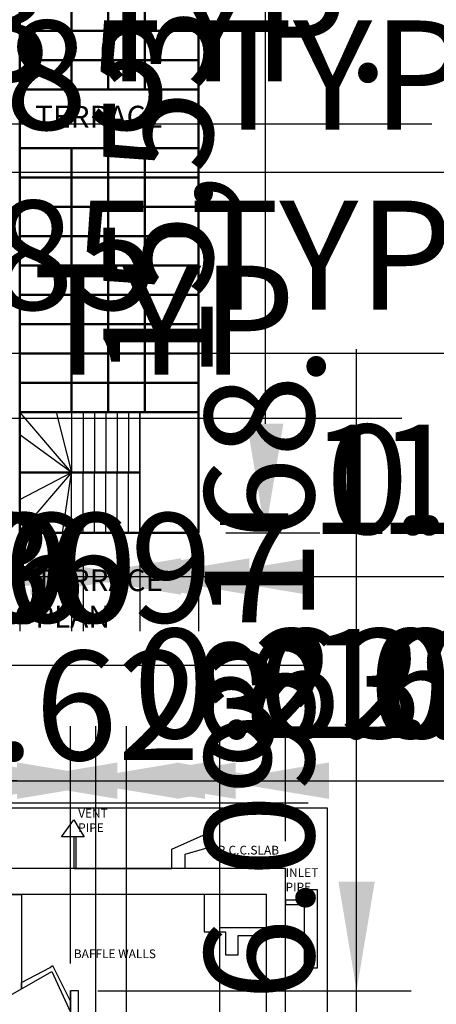
# Model space of a CAD drawing. Units: metres. Extents: x 782 to 1487, y 1262 to 7446.
# Tile 15 of 25: x 840.09 to 849.63, y 1279.51 to 1302.06. Entities that reach past the tile are written whole.
import ezdxf

# ---------------------------------------------------------------- set-up
doc = ezdxf.new("R2010")
doc.units = ezdxf.units.M
for name, color, linetype, lineweight in [('A-ANNO-DIMS', 2, 'Continuous', 18), ('A-ANNO-TEXT', 3, 'Continuous', 18), ('A-AREA-IDEN', 3, 'Continuous', 18), ('A-DETL', 7, 'Continuous', 25), ('A-FLOR-STRS', 3, 'Continuous', 25), ('A-WALL', 7, 'Continuous', 50)]:
    doc.layers.add(name, color=color, linetype=linetype, lineweight=lineweight)
doc.styles.get("Standard").update_dxf_attribs({"font": 'arial.ttf'})
doc.dimstyles.new('ISO-25', dxfattribs={"dimtxt": 2.5, "dimasz": 2.5, "dimexe": 1.25, "dimexo": 0.625, "dimtad": 1, "dimtxsty": 'Standard', "dimcen": 2.5, "dimadec": 0, "dimazin": 0, "dimtfac": 1, "dimtmove": 0, "dimatfit": 3, "dimfxl": 1, "dimarcsym": 0})

# ---------------------------------------------------------------- blocks, each defined once
blk = doc.blocks.new('*D8')
at = {"layer": 'A-ANNO-DIMS', "color": 0, "lineweight": -2, "transparency": 16777216}
for p, q in [((844.81, 1305.835), (846.96, 1305.835)), ((845.71, 1303.335), (845.71, 1292.805)), ((844.81, 1290.305), (846.96, 1290.305))]:
    blk.add_line(p, q, dxfattribs=at)
at = {"layer": 'A-ANNO-DIMS', "color": 0, "transparency": 16777216}
for points in [[(845.293, 1303.335), (846.126, 1303.335), (845.71, 1305.835)], [(845.293, 1292.805), (846.126, 1292.805), (845.71, 1290.305)]]:
    blk.add_solid(points, dxfattribs=at)
at = {"layer": 'Defpoints', "color": 0, "transparency": 16777216}
for p in [(844.185, 1305.835), (844.185, 1290.305), (845.71, 1290.305)]:
    blk.add_point(p, dxfattribs=at)
at = {"layer": 'A-ANNO-DIMS', "color": 0, "transparency": 16777216, "insert": (843.582, 1298.07), "char_height": 2.5, "attachment_point": 5, "rotation": 90}
blk.add_mtext('15,53', dxfattribs=at)
blk = doc.blocks.new('*D21')
at = {"layer": 'A-ANNO-DIMS', "color": 0, "lineweight": -2, "transparency": 16777216}
for p, q in [((827.576, 1298.565), (825.076, 1298.565)), ((830.076, 1298.565), (830.923, 1298.565)), ((833.423, 1298.565), (852.255, 1298.565)), ((830.076, 1298.073), (830.076, 1297.315)), ((830.923, 1298.073), (830.923, 1297.315))]:
    blk.add_line(p, q, dxfattribs=at)
at = {"layer": 'A-ANNO-DIMS', "color": 0, "transparency": 16777216}
for points in [[(827.576, 1298.981), (827.576, 1298.148), (830.076, 1298.565)], [(833.423, 1298.981), (833.423, 1298.148), (830.923, 1298.565)]]:
    blk.add_solid(points, dxfattribs=at)
at = {"layer": 'Defpoints', "color": 0, "transparency": 16777216}
for p in [(830.076, 1298.698), (830.923, 1298.698), (830.923, 1298.565)]:
    blk.add_point(p, dxfattribs=at)
at = {"layer": 'A-ANNO-DIMS', "color": 0, "transparency": 16777216, "insert": (844.089, 1300.466), "char_height": 2.5, "attachment_point": 5}
blk.add_mtext('0.85 TYP.', dxfattribs=at)
blk = doc.blocks.new('*D22')
at = {"layer": 'A-ANNO-DIMS', "color": 0, "lineweight": -2, "transparency": 16777216}
for p, q in [((812.79, 1292.934), (810.29, 1292.934)), ((815.29, 1292.934), (816.179, 1292.934)), ((818.679, 1292.934), (848.834, 1292.934)), ((815.29, 1292.442), (815.29, 1291.684)), ((816.179, 1292.442), (816.179, 1291.684))]:
    blk.add_line(p, q, dxfattribs=at)
at = {"layer": 'A-ANNO-DIMS', "color": 0, "transparency": 16777216}
for points in [[(812.79, 1293.351), (812.79, 1292.517), (815.29, 1292.934)], [(818.679, 1293.351), (818.679, 1292.517), (816.179, 1292.934)]]:
    blk.add_solid(points, dxfattribs=at)
at = {"layer": 'Defpoints', "color": 0, "transparency": 16777216}
for p in [(815.29, 1293.067), (816.179, 1293.067), (816.179, 1292.934)]:
    blk.add_point(p, dxfattribs=at)
at = {"layer": 'A-ANNO-DIMS', "color": 0, "transparency": 16777216, "insert": (835.007, 1294.852), "char_height": 2.5, "attachment_point": 5}
blk.add_mtext('DOOR 0.89 TYP.', dxfattribs=at)
blk = doc.blocks.new('*D24')
at = {"layer": 'A-ANNO-DIMS', "color": 0, "lineweight": -2, "transparency": 16777216}
for p, q in [((811.209, 1294.423), (808.709, 1294.423)), ((813.709, 1294.423), (814.559, 1294.423)), ((817.059, 1294.423), (852.649, 1294.423)), ((813.709, 1293.926), (813.709, 1293.173)), ((814.559, 1293.926), (814.559, 1293.173))]:
    blk.add_line(p, q, dxfattribs=at)
at = {"layer": 'A-ANNO-DIMS', "color": 0, "transparency": 16777216}
for points in [[(811.209, 1294.84), (811.209, 1294.006), (813.709, 1294.423)], [(817.059, 1294.84), (817.059, 1294.006), (814.559, 1294.423)]]:
    blk.add_solid(points, dxfattribs=at)
at = {"layer": 'Defpoints', "color": 0, "transparency": 16777216}
for p in [(813.709, 1294.551), (814.559, 1294.551), (814.559, 1294.423)]:
    blk.add_point(p, dxfattribs=at)
at = {"layer": 'A-ANNO-DIMS', "color": 0, "transparency": 16777216, "insert": (836.104, 1296.342), "char_height": 2.5, "attachment_point": 5}
blk.add_mtext('DOOR D2 0.85 TYP.', dxfattribs=at)
blk = doc.blocks.new('*D27')
at = {"layer": 'A-ANNO-DIMS', "color": 0, "lineweight": -2, "transparency": 16777216}
for p, q in [((825.463, 1299.672), (822.963, 1299.672)), ((827.963, 1299.672), (828.193, 1299.672)), ((830.693, 1299.672), (849.525, 1299.672)), ((827.963, 1299.184), (827.963, 1298.422)), ((828.193, 1299.184), (828.193, 1298.422))]:
    blk.add_line(p, q, dxfattribs=at)
at = {"layer": 'A-ANNO-DIMS', "color": 0, "transparency": 16777216}
for points in [[(825.463, 1300.088), (825.463, 1299.255), (827.963, 1299.672)], [(830.693, 1300.088), (830.693, 1299.255), (828.193, 1299.672)]]:
    blk.add_solid(points, dxfattribs=at)
at = {"layer": 'Defpoints', "color": 0, "transparency": 16777216}
for p in [(827.963, 1299.809), (828.193, 1299.809), (828.193, 1299.672)]:
    blk.add_point(p, dxfattribs=at)
at = {"layer": 'A-ANNO-DIMS', "color": 0, "transparency": 16777216, "insert": (841.359, 1301.574), "char_height": 2.5, "attachment_point": 5}
blk.add_mtext('0.23 TYP.', dxfattribs=at)
blk = doc.blocks.new('*D97')
at = {"layer": 'A-ANNO-DIMS', "color": 0, "lineweight": -2, "transparency": 16777216}
for p, q in [((827.962, 1289.68), (827.962, 1286.027)), ((829.151, 1289.68), (829.151, 1286.027)), ((825.462, 1287.277), (822.962, 1287.277)), ((827.962, 1287.277), (829.151, 1287.277)), ((831.651, 1287.277), (841.665, 1287.277))]:
    blk.add_line(p, q, dxfattribs=at)
at = {"layer": 'A-ANNO-DIMS', "color": 0, "transparency": 16777216}
for points in [[(825.462, 1287.694), (825.462, 1286.861), (827.962, 1287.277)], [(831.651, 1287.694), (831.651, 1286.861), (829.151, 1287.277)]]:
    blk.add_solid(points, dxfattribs=at)
at = {"layer": 'Defpoints', "color": 0, "transparency": 16777216}
for p in [(827.962, 1290.305), (829.151, 1290.305), (829.151, 1287.277)]:
    blk.add_point(p, dxfattribs=at)
at = {"layer": 'A-ANNO-DIMS', "color": 0, "transparency": 16777216, "insert": (837.908, 1289.179), "char_height": 2.5, "attachment_point": 5}
blk.add_mtext('1.19', dxfattribs=at)
blk = doc.blocks.new('*D98')
at = {"layer": 'A-ANNO-DIMS', "color": 0, "lineweight": -2, "transparency": 16777216}
for p, q in [((829.151, 1289.68), (829.151, 1286.027)), ((829.412, 1289.68), (829.412, 1286.027)), ((826.651, 1287.277), (824.151, 1287.277)), ((829.151, 1287.277), (829.412, 1287.277)), ((831.912, 1287.277), (842.154, 1287.277))]:
    blk.add_line(p, q, dxfattribs=at)
at = {"layer": 'A-ANNO-DIMS', "color": 0, "transparency": 16777216}
for points in [[(826.651, 1287.694), (826.651, 1286.861), (829.151, 1287.277)], [(831.912, 1287.694), (831.912, 1286.861), (829.412, 1287.277)]]:
    blk.add_solid(points, dxfattribs=at)
at = {"layer": 'Defpoints', "color": 0, "transparency": 16777216}
for p in [(829.151, 1290.305), (829.412, 1290.305), (829.412, 1287.277)]:
    blk.add_point(p, dxfattribs=at)
at = {"layer": 'A-ANNO-DIMS', "color": 0, "transparency": 16777216, "insert": (838.283, 1289.179), "char_height": 2.5, "attachment_point": 5}
blk.add_mtext('0.26', dxfattribs=at)
blk = doc.blocks.new('*D99')
at = {"layer": 'A-ANNO-DIMS', "color": 0, "lineweight": -2, "transparency": 16777216}
for p, q in [((829.412, 1289.68), (829.412, 1286.027)), ((830.716, 1289.68), (830.716, 1286.027)), ((826.912, 1287.277), (824.412, 1287.277)), ((829.412, 1287.277), (830.716, 1287.277)), ((833.216, 1287.277), (843.216, 1287.277))]:
    blk.add_line(p, q, dxfattribs=at)
at = {"layer": 'A-ANNO-DIMS', "color": 0, "transparency": 16777216}
for points in [[(826.912, 1287.694), (826.912, 1286.861), (829.412, 1287.277)], [(833.216, 1287.694), (833.216, 1286.861), (830.716, 1287.277)]]:
    blk.add_solid(points, dxfattribs=at)
at = {"layer": 'Defpoints', "color": 0, "transparency": 16777216}
for p in [(829.412, 1290.305), (830.716, 1290.305), (830.716, 1287.277)]:
    blk.add_point(p, dxfattribs=at)
at = {"layer": 'A-ANNO-DIMS', "color": 0, "transparency": 16777216, "insert": (839.466, 1289.18), "char_height": 2.5, "attachment_point": 5}
blk.add_mtext('1.30', dxfattribs=at)
blk = doc.blocks.new('*D100')
at = {"layer": 'A-ANNO-DIMS', "color": 0, "lineweight": -2, "transparency": 16777216}
for p, q in [((830.716, 1289.68), (830.716, 1286.027)), ((832.412, 1289.68), (832.412, 1286.027)), ((828.216, 1287.277), (825.716, 1287.277)), ((830.716, 1287.277), (832.412, 1287.277)), ((834.912, 1287.277), (846.863, 1287.277))]:
    blk.add_line(p, q, dxfattribs=at)
at = {"layer": 'A-ANNO-DIMS', "color": 0, "transparency": 16777216}
for points in [[(828.216, 1287.694), (828.216, 1286.861), (830.716, 1287.277)], [(834.912, 1287.694), (834.912, 1286.861), (832.412, 1287.277)]]:
    blk.add_solid(points, dxfattribs=at)
at = {"layer": 'Defpoints', "color": 0, "transparency": 16777216}
for p in [(830.716, 1290.305), (832.412, 1290.305), (832.412, 1287.277)]:
    blk.add_point(p, dxfattribs=at)
at = {"layer": 'A-ANNO-DIMS', "color": 0, "transparency": 16777216, "insert": (842.138, 1289.179), "char_height": 2.5, "attachment_point": 5}
blk.add_mtext('1.697', dxfattribs=at)
blk = doc.blocks.new('*D105')
at = {"layer": 'A-ANNO-DIMS', "color": 0, "lineweight": -2, "transparency": 16777216}
for p, q in [((840.091, 1289.68), (840.091, 1288.055)), ((841.28, 1289.68), (841.28, 1288.055)), ((837.591, 1289.305), (835.091, 1289.305)), ((840.091, 1289.305), (841.28, 1289.305)), ((843.78, 1289.305), (853.794, 1289.305))]:
    blk.add_line(p, q, dxfattribs=at)
at = {"layer": 'A-ANNO-DIMS', "color": 0, "transparency": 16777216}
for points in [[(837.591, 1289.722), (837.591, 1288.889), (840.091, 1289.305)], [(843.78, 1289.722), (843.78, 1288.889), (841.28, 1289.305)]]:
    blk.add_solid(points, dxfattribs=at)
at = {"layer": 'Defpoints', "color": 0, "transparency": 16777216}
for p in [(840.091, 1290.305), (841.28, 1290.305), (841.28, 1289.305)]:
    blk.add_point(p, dxfattribs=at)
at = {"layer": 'A-ANNO-DIMS', "color": 0, "transparency": 16777216, "insert": (850.037, 1291.207), "char_height": 2.5, "attachment_point": 5}
blk.add_mtext('1.19', dxfattribs=at)
blk = doc.blocks.new('*D106')
at = {"layer": 'A-ANNO-DIMS', "color": 0, "lineweight": -2, "transparency": 16777216}
for p, q in [((841.28, 1289.68), (841.28, 1288.055)), ((841.541, 1289.68), (841.541, 1288.055)), ((838.78, 1289.305), (836.28, 1289.305)), ((841.28, 1289.305), (841.541, 1289.305)), ((844.041, 1289.305), (854.283, 1289.305))]:
    blk.add_line(p, q, dxfattribs=at)
at = {"layer": 'A-ANNO-DIMS', "color": 0, "transparency": 16777216}
for points in [[(838.78, 1289.722), (838.78, 1288.889), (841.28, 1289.305)], [(844.041, 1289.722), (844.041, 1288.889), (841.541, 1289.305)]]:
    blk.add_solid(points, dxfattribs=at)
at = {"layer": 'Defpoints', "color": 0, "transparency": 16777216}
for p in [(841.28, 1290.305), (841.541, 1290.305), (841.541, 1289.305)]:
    blk.add_point(p, dxfattribs=at)
at = {"layer": 'A-ANNO-DIMS', "color": 0, "transparency": 16777216, "insert": (850.412, 1291.207), "char_height": 2.5, "attachment_point": 5}
blk.add_mtext('0.26', dxfattribs=at)
blk = doc.blocks.new('*D107')
at = {"layer": 'A-ANNO-DIMS', "color": 0, "lineweight": -2, "transparency": 16777216}
for p, q in [((841.541, 1289.68), (841.541, 1288.055)), ((842.844, 1289.68), (842.844, 1288.055)), ((839.041, 1289.305), (836.541, 1289.305)), ((841.541, 1289.305), (842.844, 1289.305)), ((845.344, 1289.305), (855.344, 1289.305))]:
    blk.add_line(p, q, dxfattribs=at)
at = {"layer": 'A-ANNO-DIMS', "color": 0, "transparency": 16777216}
for points in [[(839.041, 1289.722), (839.041, 1288.889), (841.541, 1289.305)], [(845.344, 1289.722), (845.344, 1288.889), (842.844, 1289.305)]]:
    blk.add_solid(points, dxfattribs=at)
at = {"layer": 'Defpoints', "color": 0, "transparency": 16777216}
for p in [(841.541, 1290.305), (842.844, 1290.305), (842.844, 1289.305)]:
    blk.add_point(p, dxfattribs=at)
at = {"layer": 'A-ANNO-DIMS', "color": 0, "transparency": 16777216, "insert": (851.594, 1291.208), "char_height": 2.5, "attachment_point": 5}
blk.add_mtext('1.30', dxfattribs=at)
blk = doc.blocks.new('*D108')
at = {"layer": 'A-ANNO-DIMS', "color": 0, "lineweight": -2, "transparency": 16777216}
for p, q in [((842.844, 1289.68), (842.844, 1288.055)), ((844.185, 1289.68), (844.185, 1288.055)), ((840.344, 1289.305), (837.844, 1289.305)), ((842.844, 1289.305), (844.185, 1289.305)), ((846.685, 1289.305), (856.683, 1289.305))]:
    blk.add_line(p, q, dxfattribs=at)
at = {"layer": 'A-ANNO-DIMS', "color": 0, "transparency": 16777216}
for points in [[(840.344, 1289.722), (840.344, 1288.889), (842.844, 1289.305)], [(846.685, 1289.722), (846.685, 1288.889), (844.185, 1289.305)]]:
    blk.add_solid(points, dxfattribs=at)
at = {"layer": 'Defpoints', "color": 0, "transparency": 16777216}
for p in [(842.844, 1290.305), (844.185, 1290.305), (844.185, 1289.305)]:
    blk.add_point(p, dxfattribs=at)
at = {"layer": 'A-ANNO-DIMS', "color": 0, "transparency": 16777216, "insert": (852.934, 1291.208), "char_height": 2.5, "attachment_point": 5}
blk.add_mtext('1.34', dxfattribs=at)
blk = doc.blocks.new('*D148')
at = {"layer": 'A-ANNO-DIMS', "color": 0, "lineweight": -2, "transparency": 16777216}
for p, q in [((847.802, 1276.491), (847.802, 1288.69)), ((846.368, 1273.991), (849.052, 1273.991)), ((847.802, 1267.897), (847.802, 1273.991)), ((846.368, 1267.897), (849.052, 1267.897)), ((847.802, 1265.397), (847.802, 1262.897))]:
    blk.add_line(p, q, dxfattribs=at)
at = {"layer": 'A-ANNO-DIMS', "color": 0, "transparency": 16777216}
for points in [[(847.386, 1276.491), (848.219, 1276.491), (847.802, 1273.991)], [(847.386, 1265.397), (848.219, 1265.397), (847.802, 1267.897)]]:
    blk.add_solid(points, dxfattribs=at)
at = {"layer": 'Defpoints', "color": 0, "transparency": 16777216}
for p in [(845.743, 1273.991), (847.802, 1273.991), (845.743, 1267.897)]:
    blk.add_point(p, dxfattribs=at)
at = {"layer": 'A-ANNO-DIMS', "color": 0, "transparency": 16777216, "insert": (845.9, 1283.841), "char_height": 2.5, "attachment_point": 5, "rotation": 90}
blk.add_mtext('6.093', dxfattribs=at)
blk = doc.blocks.new('*D151')
at = {"layer": 'A-ANNO-DIMS', "color": 0, "lineweight": -2, "transparency": 16777216}
for p, q in [((839.686, 1273.694), (839.686, 1285.879)), ((841.835, 1273.694), (841.835, 1285.879)), ((837.186, 1284.629), (834.686, 1284.629)), ((839.686, 1284.629), (841.835, 1284.629)), ((844.335, 1284.629), (856.569, 1284.629))]:
    blk.add_line(p, q, dxfattribs=at)
at = {"layer": 'A-ANNO-DIMS', "color": 0, "transparency": 16777216}
for points in [[(837.186, 1285.046), (837.186, 1284.212), (839.686, 1284.629)], [(844.335, 1285.046), (844.335, 1284.212), (841.835, 1284.629)]]:
    blk.add_solid(points, dxfattribs=at)
at = {"layer": 'Defpoints', "color": 0, "transparency": 16777216}
for p in [(841.835, 1284.629), (839.686, 1273.069), (841.835, 1273.069)]:
    blk.add_point(p, dxfattribs=at)
at = {"layer": 'A-ANNO-DIMS', "color": 0, "transparency": 16777216, "insert": (851.702, 1286.531), "char_height": 2.5, "attachment_point": 5}
blk.add_mtext('2.149', dxfattribs=at)
blk = doc.blocks.new('*D152')
at = {"layer": 'A-ANNO-DIMS', "color": 0, "lineweight": -2, "transparency": 16777216}
for p, q in [((841.835, 1273.694), (841.835, 1285.879)), ((842.533, 1273.678), (842.533, 1285.879)), ((839.335, 1284.629), (836.835, 1284.629)), ((841.835, 1284.629), (842.533, 1284.629)), ((845.033, 1284.629), (855.269, 1284.629))]:
    blk.add_line(p, q, dxfattribs=at)
at = {"layer": 'A-ANNO-DIMS', "color": 0, "transparency": 16777216}
for points in [[(839.335, 1285.046), (839.335, 1284.212), (841.835, 1284.629)], [(845.033, 1285.046), (845.033, 1284.212), (842.533, 1284.629)]]:
    blk.add_solid(points, dxfattribs=at)
at = {"layer": 'Defpoints', "color": 0, "transparency": 16777216}
for p in [(842.533, 1284.629), (841.835, 1273.069), (842.533, 1273.053)]:
    blk.add_point(p, dxfattribs=at)
at = {"layer": 'A-ANNO-DIMS', "color": 0, "transparency": 16777216, "insert": (851.401, 1286.531), "char_height": 2.5, "attachment_point": 5}
blk.add_mtext('0.70', dxfattribs=at)
blk = doc.blocks.new('*D153')
at = {"layer": 'A-ANNO-DIMS', "color": 0, "lineweight": -2, "transparency": 16777216}
for p, q in [((842.533, 1273.678), (842.533, 1285.879)), ((844.669, 1273.698), (844.669, 1285.879)), ((840.033, 1284.629), (837.533, 1284.629)), ((842.533, 1284.629), (844.669, 1284.629)), ((847.169, 1284.629), (857.445, 1284.629))]:
    blk.add_line(p, q, dxfattribs=at)
at = {"layer": 'A-ANNO-DIMS', "color": 0, "transparency": 16777216}
for points in [[(840.033, 1285.046), (840.033, 1284.212), (842.533, 1284.629)], [(847.169, 1285.046), (847.169, 1284.212), (844.669, 1284.629)]]:
    blk.add_solid(points, dxfattribs=at)
at = {"layer": 'Defpoints', "color": 0, "transparency": 16777216}
for p in [(844.669, 1284.629), (842.533, 1273.053), (844.669, 1273.073)]:
    blk.add_point(p, dxfattribs=at)
at = {"layer": 'A-ANNO-DIMS', "color": 0, "transparency": 16777216, "insert": (853.557, 1286.509), "char_height": 2.5, "attachment_point": 5}
blk.add_mtext('2.14', dxfattribs=at)
blk = doc.blocks.new('*D156')
at = {"layer": 'A-ANNO-DIMS', "color": 0, "lineweight": -2, "transparency": 16777216}
for p, q in [((836.503, 1283.244), (836.503, 1285.879)), ((846.176, 1283.244), (846.176, 1285.879)), ((839.003, 1284.629), (843.676, 1284.629)), ((846.176, 1284.629), (858.362, 1284.629))]:
    blk.add_line(p, q, dxfattribs=at)
at = {"layer": 'A-ANNO-DIMS', "color": 0, "transparency": 16777216}
for points in [[(839.003, 1285.046), (839.003, 1284.212), (836.503, 1284.629)], [(843.676, 1285.046), (843.676, 1284.212), (846.176, 1284.629)]]:
    blk.add_solid(points, dxfattribs=at)
at = {"layer": 'Defpoints', "color": 0, "transparency": 16777216}
for p in [(846.176, 1284.629), (836.503, 1282.619), (846.176, 1282.619)]:
    blk.add_point(p, dxfattribs=at)
at = {"layer": 'A-ANNO-DIMS', "color": 0, "transparency": 16777216, "insert": (853.519, 1286.531), "char_height": 2.5, "attachment_point": 5}
blk.add_mtext('9.673', dxfattribs=at)
blk = doc.blocks.new('*D158')
at = {"layer": 'A-ANNO-DIMS', "color": 0, "lineweight": -2, "transparency": 16777216}
for p, q in [((836.503, 1283.244), (836.503, 1285.879)), ((837.132, 1282.644), (837.132, 1285.879)), ((834.003, 1284.629), (831.503, 1284.629)), ((836.503, 1284.629), (837.132, 1284.629)), ((839.632, 1284.629), (849.876, 1284.629))]:
    blk.add_line(p, q, dxfattribs=at)
at = {"layer": 'A-ANNO-DIMS', "color": 0, "transparency": 16777216}
for points in [[(834.003, 1285.046), (834.003, 1284.212), (836.503, 1284.629)], [(839.632, 1285.046), (839.632, 1284.212), (837.132, 1284.629)]]:
    blk.add_solid(points, dxfattribs=at)
at = {"layer": 'Defpoints', "color": 0, "transparency": 16777216}
for p in [(837.132, 1284.629), (836.503, 1282.619), (837.132, 1282.019)]:
    blk.add_point(p, dxfattribs=at)
at = {"layer": 'A-ANNO-DIMS', "color": 0, "transparency": 16777216, "insert": (846.004, 1286.531), "char_height": 2.5, "attachment_point": 5}
blk.add_mtext('0.63', dxfattribs=at)
blk = doc.blocks.new('*D159')
at = {"layer": 'A-ANNO-DIMS', "color": 0, "lineweight": -2, "transparency": 16777216}
for p, q in [((837.132, 1282.644), (837.132, 1285.879)), ((839.826, 1282.644), (839.826, 1285.879)), ((834.632, 1284.629), (832.132, 1284.629)), ((837.132, 1284.629), (839.826, 1284.629)), ((842.326, 1284.629), (854.545, 1284.629))]:
    blk.add_line(p, q, dxfattribs=at)
at = {"layer": 'A-ANNO-DIMS', "color": 0, "transparency": 16777216}
for points in [[(834.632, 1285.046), (834.632, 1284.212), (837.132, 1284.629)], [(842.326, 1285.046), (842.326, 1284.212), (839.826, 1284.629)]]:
    blk.add_solid(points, dxfattribs=at)
at = {"layer": 'Defpoints', "color": 0, "transparency": 16777216}
for p in [(839.826, 1284.629), (837.132, 1282.019), (839.826, 1282.019)]:
    blk.add_point(p, dxfattribs=at)
at = {"layer": 'A-ANNO-DIMS', "color": 0, "transparency": 16777216, "insert": (849.686, 1286.531), "char_height": 2.5, "attachment_point": 5}
blk.add_mtext('2.694', dxfattribs=at)
blk = doc.blocks.new('*D160')
at = {"layer": 'A-ANNO-DIMS', "color": 0, "lineweight": -2, "transparency": 16777216}
for p, q in [((839.826, 1280.313), (839.826, 1285.879)), ((841.255, 1280.444), (841.255, 1285.879)), ((837.326, 1284.629), (834.826, 1284.629)), ((839.826, 1284.629), (841.255, 1284.629)), ((843.755, 1284.629), (853.764, 1284.629))]:
    blk.add_line(p, q, dxfattribs=at)
at = {"layer": 'A-ANNO-DIMS', "color": 0, "transparency": 16777216}
for points in [[(837.326, 1285.046), (837.326, 1284.212), (839.826, 1284.629)], [(843.755, 1285.046), (843.755, 1284.212), (841.255, 1284.629)]]:
    blk.add_solid(points, dxfattribs=at)
at = {"layer": 'Defpoints', "color": 0, "transparency": 16777216}
for p in [(841.255, 1284.629), (841.255, 1279.819), (839.826, 1279.688)]:
    blk.add_point(p, dxfattribs=at)
at = {"layer": 'A-ANNO-DIMS', "color": 0, "transparency": 16777216, "insert": (850.01, 1286.531), "char_height": 2.5, "attachment_point": 5}
blk.add_mtext('1.43', dxfattribs=at)
blk = doc.blocks.new('*D161')
at = {"layer": 'A-ANNO-DIMS', "color": 0, "lineweight": -2, "transparency": 16777216}
for p, q in [((847.802, 1282.319), (847.802, 1294.509)), ((841.88, 1279.819), (849.052, 1279.819)), ((847.802, 1276.651), (847.802, 1279.819)), ((841.88, 1276.651), (849.052, 1276.651)), ((847.802, 1274.151), (847.802, 1271.651))]:
    blk.add_line(p, q, dxfattribs=at)
at = {"layer": 'A-ANNO-DIMS', "color": 0, "transparency": 16777216}
for points in [[(847.386, 1282.319), (848.219, 1282.319), (847.802, 1279.819)], [(847.386, 1274.151), (848.219, 1274.151), (847.802, 1276.651)]]:
    blk.add_solid(points, dxfattribs=at)
at = {"layer": 'Defpoints', "color": 0, "transparency": 16777216}
for p in [(841.255, 1279.819), (847.802, 1279.819), (841.255, 1276.651)]:
    blk.add_point(p, dxfattribs=at)
at = {"layer": 'A-ANNO-DIMS', "color": 0, "transparency": 16777216, "insert": (845.9, 1289.664), "char_height": 2.5, "attachment_point": 5, "rotation": 90}
blk.add_mtext('3.168', dxfattribs=at)
blk = doc.blocks.new('*D165')
at = {"layer": 'A-ANNO-DIMS', "color": 0, "lineweight": -2, "transparency": 16777216}
for p, q in [((826.388, 1283.885), (826.388, 1285.375)), ((832.011, 1283.885), (832.011, 1285.375)), ((823.888, 1284.125), (821.388, 1284.125)), ((826.388, 1284.125), (832.011, 1284.125)), ((834.511, 1284.125), (846.697, 1284.125))]:
    blk.add_line(p, q, dxfattribs=at)
at = {"layer": 'A-ANNO-DIMS', "color": 0, "transparency": 16777216}
for points in [[(823.888, 1284.541), (823.888, 1283.708), (826.388, 1284.125)], [(834.511, 1284.541), (834.511, 1283.708), (832.011, 1284.125)]]:
    blk.add_solid(points, dxfattribs=at)
at = {"layer": 'Defpoints', "color": 0, "transparency": 16777216}
for p in [(832.011, 1284.125), (826.388, 1283.26), (832.011, 1283.26)]:
    blk.add_point(p, dxfattribs=at)
at = {"layer": 'A-ANNO-DIMS', "color": 0, "transparency": 16777216, "insert": (841.854, 1286.027), "char_height": 2.5, "attachment_point": 5}
blk.add_mtext('5.623', dxfattribs=at)

msp = doc.modelspace()

# ---------------------------------------------------------------- linework, layer by layer
at = {"layer": 'A-DETL'}
for p, q in [((841.0475, 1283.3454), (841.3293, 1283.7291)), ((841.3293, 1283.7291), (841.4773, 1283.491)), ((841.3396, 1283.3454), (841.0475, 1283.3454)), ((841.3396, 1282.619), (841.3396, 1283.3454)), ((841.5677, 1283.3454), (841.3396, 1283.3454)), ((841.3807, 1282.619), (841.3807, 1283.3454)), ((841.4773, 1283.491), (841.5677, 1283.3454)), ((843.5698, 1283.0622), (844.4285, 1283.4455)), ((844.4285, 1283.4455), (844.4285, 1283.0987)), ((843.5698, 1282.619), (843.5698, 1283.0622)), ((844.4285, 1283.0987), (843.8731, 1282.9355)), ((843.8731, 1282.9355), (843.8731, 1282.619)), ((841.3396, 1282.619), (843.5698, 1282.619)), ((841.3396, 1282.619), (841.5184, 1282.619)), ((841.5184, 1282.619), (841.3807, 1282.619)), ((841.4362, 1282.0186), (839.8262, 1282.0186)), ((839.8262, 1282.0186), (840.1341, 1282.0186)), ((840.1341, 1282.0186), (840.1341, 1279.8643)), ((845.7402, 1282.0186), (844.3095, 1282.0186)), ((844.3095, 1282.0186), (844.3095, 1281.1685)), ((844.673, 1281.2573), (844.673, 1282.0186)), ((846.6099, 1282.1389), (846.9023, 1282.1389)), ((846.6099, 1280.3321), (846.6099, 1282.1389)), ((846.6099, 1282.1389), (846.6099, 1281.8914)), ((846.9023, 1282.1389), (846.9023, 1280.3321)), ((846.6099, 1281.8914), (846.1759, 1281.8914)), ((846.1759, 1281.8914), (846.1759, 1281.7954)), ((846.1759, 1281.7954), (846.6099, 1281.7954)), ((846.6099, 1281.7954), (846.6099, 1281.8914)), ((844.3095, 1281.1685), (844.8002, 1281.1685)), ((845.7402, 1281.2573), (844.673, 1281.2573)), ((844.8002, 1281.1685), (844.8002, 1280.6419)), ((845.0943, 1280.6419), (845.0943, 1281.0866)), ((845.0943, 1281.0866), (845.7402, 1281.0866)), ((845.7402, 1281.0866), (845.7402, 1281.2573)), ((844.8002, 1280.6419), (845.0943, 1280.6419)), ((839.8262, 1279.6878), (840.8283, 1280.2623)), ((840.1341, 1280.0091), (840.7874, 1280.352)), ((840.7874, 1280.352), (840.8402, 1280.3927)), ((840.8283, 1280.2623), (841.2554, 1279.3267)), ((840.8402, 1280.3927), (841.2554, 1279.5729)), ((846.9023, 1280.3321), (846.6099, 1280.3321)), ((840.1341, 1279.8643), (840.1341, 1280.0091)), ((841.2554, 1279.3267), (841.2554, 1279.8192)), ((841.2554, 1279.8192), (841.2554, 1276.6513)), ((841.4362, 1279.8192), (841.2554, 1279.8192)), ((841.4362, 1276.6513), (841.4362, 1279.8192))]:
    msp.add_line(p, q, dxfattribs=at)
for points in [[(823.6278, 1284.0012), (823.6278, 1266.59), (847.1334, 1266.59), (847.1334, 1284.0012)], [(836.5033, 1282.619), (836.5033, 1276.2022), (846.1759, 1276.2022), (846.1759, 1282.619)], [(837.1321, 1282.0186), (837.1321, 1276.6513), (845.7402, 1276.6513), (845.7402, 1282.0186)]]:
    msp.add_lwpolyline(points, close=True, dxfattribs=at)
at = {"layer": 'A-FLOR-STRS'}
for p, q in [((841.2801, 1291.6863), (840.0913, 1293.0674)), ((840.9263, 1293.0674), (841.2801, 1291.6863)), ((841.2801, 1293.0674), (841.2801, 1291.6863)), ((841.5409, 1293.0674), (841.5409, 1291.6863)), ((841.8016, 1293.0674), (841.8016, 1291.6863)), ((842.0623, 1293.0674), (842.0623, 1291.6863)), ((842.323, 1293.0674), (842.323, 1291.6863)), ((842.5837, 1293.0674), (842.5837, 1291.6863)), ((842.8445, 1290.3053), (842.8445, 1293.0674)), ((842.8445, 1293.0674), (842.8445, 1290.3053)), ((842.8445, 1293.0674), (842.8445, 1291.6863)), ((841.2801, 1291.6863), (840.0913, 1292.5526)), ((841.2801, 1291.6863), (840.0913, 1290.3053)), ((841.2801, 1291.6863), (840.0913, 1291.6863)), ((840.0913, 1291.0666), (841.2801, 1291.6863)), ((841.0721, 1290.3053), (841.2801, 1291.6863)), ((841.2801, 1290.3053), (841.2801, 1291.6863)), ((841.5409, 1290.3053), (841.5409, 1291.6863)), ((841.8016, 1290.3053), (841.8016, 1291.6863)), ((842.0623, 1290.3053), (842.0623, 1291.6863)), ((842.323, 1290.3053), (842.323, 1291.6863)), ((842.5837, 1290.3053), (842.5837, 1291.6863)), ((842.8445, 1290.3053), (842.8445, 1291.6863))]:
    msp.add_line(p, q, dxfattribs=at)
at = {"layer": 'A-WALL'}
for p, q in [((840.0949, 1305.8353), (840.0949, 1290.3053)), ((841.2801, 1300.4593), (841.2801, 1305.8353)), ((842.1182, 1305.8353), (842.1182, 1300.4593)), ((842.9563, 1305.8353), (842.9563, 1300.4593)), ((844.1849, 1290.3053), (844.1849, 1305.8353)), ((840.0913, 1301.8033), (844.1849, 1301.8033)), ((840.0913, 1301.1313), (844.1849, 1301.1313)), ((840.0913, 1300.4593), (844.1849, 1300.4593)), ((840.0913, 1299.7873), (840.0949, 1299.7873)), ((840.0913, 1299.1153), (844.1849, 1299.1153)), ((841.2801, 1293.0674), (841.2801, 1299.1153)), ((842.1182, 1299.1153), (842.1182, 1293.0674)), ((842.9563, 1299.1153), (842.9563, 1293.0674)), ((840.0913, 1298.4434), (844.1849, 1298.4434)), ((840.0913, 1297.7714), (844.1849, 1297.7714)), ((840.0913, 1297.0994), (844.1849, 1297.0994)), ((840.0913, 1296.4274), (844.1849, 1296.4274)), ((840.0913, 1295.7554), (844.1849, 1295.7554)), ((840.0913, 1295.0834), (844.1849, 1295.0834)), ((840.0913, 1294.4114), (844.1849, 1294.4114)), ((840.0913, 1293.7394), (844.1849, 1293.7394)), ((840.0913, 1293.0674), (840.0913, 1290.3053)), ((840.0913, 1293.0674), (841.2801, 1293.0674)), ((840.0913, 1293.0674), (844.1849, 1293.0674)), ((844.1849, 1293.0674), (840.0949, 1293.0674)), ((840.0949, 1290.3053), (840.0949, 1292.989)), ((842.8445, 1291.6863), (840.0913, 1291.6863)), ((842.8445, 1291.6863), (840.0913, 1291.6863)), ((840.0913, 1291.6863), (840.0913, 1291.0666)), ((840.0913, 1290.3053), (844.1849, 1290.3053)), ((840.0913, 1290.3053), (841.0721, 1290.3053)), ((840.0949, 1290.3053), (844.1849, 1290.3053))]:
    msp.add_line(p, q, dxfattribs=at)

# ---------------------------------------------------------------- texts
at = {"layer": 'A-ANNO-TEXT', "char_height": 0.2, "attachment_point": 1}
for s, width, insert in [('\\PVENT PIPE', 0.600544, (841.4299, 1284.319)), ('\\PR.C.C.SLAB', 1.737484, (844.6225, 1283.4712)), ('\\PINLET PIPE', 0.957559, (846.1759, 1282.9585)), ('\\PBAFFLE WALLS', 2.014223, (841.3298, 1281.0979))]:
    msp.add_mtext_dynamic_manual_height_columns(s, width=width, gutter_width=12.5, heights=[0], dxfattribs=dict(at, insert=insert))
at = {"layer": 'A-AREA-IDEN', "char_height": 0.5, "attachment_point": 1}
for s, insert in [('\\PTERRACE ', (840.4456, 1300.9198)), ('\\PTERRACE  PLAN', (840.4456, 1290.303))]:
    msp.add_mtext_dynamic_manual_height_columns(s, width=3.452419, gutter_width=12.5, heights=[0], dxfattribs=dict(at, insert=insert))

# ---------------------------------------------------------------- dimensions: what is measured, and where the dimension line sits
at = {"layer": 'A-ANNO-DIMS'}
for base, p1, p2, override, picture, middle in [((845.7096, 1290.3053), (844.1849, 1305.8353), (844.1849, 1290.3053), {"dimclrd": 0, "dimclre": 0, "dimclrt": 0}, '*D8', (843.5822, 1298.0703)), ((847.8023, 1279.8192), (841.2554, 1276.6513), (841.2554, 1279.8192), {"dimdec": 3, "dimlfac": 1, "dimrnd": 0, "dimzin": 0, "dimdsep": 46, "dimlunit": 2}, '*D161', (845.9, 1289.664)), ((847.8023, 1273.99059), (845.74287, 1267.89715), (845.74287, 1273.99059), {"dimdec": 3, "dimlfac": 1, "dimrnd": 0, "dimzin": 0, "dimdsep": 46, "dimlunit": 2}, '*D148', (845.90001, 1283.84052))]:
    dim = msp.add_linear_dim(base=base, p1=p1, p2=p2, angle=90, dimstyle='ISO-25', override=override, dxfattribs=at)
    dim.commit()
    dim.dimension.update_dxf_attribs({"geometry": picture, "text_midpoint": middle})
for base, p1, p2, text, picture, middle in [((828.1931, 1299.6717), (827.9631, 1299.8088), (828.1931, 1299.8088), '<> TYP.', '*D27', (841.359, 1301.574)), ((814.5592, 1294.4231), (813.7086, 1294.5507), (814.5592, 1294.5507), 'DOOR D2 <> TYP.', '*D24', (836.1042, 1296.3416)), ((830.923, 1298.5648), (830.0763, 1298.6982), (830.923, 1298.6982), '<> TYP.', '*D21', (844.0889, 1300.4662)), ((816.1792, 1292.934), (815.2897, 1293.0674), (816.1792, 1293.0674), 'DOOR <> TYP.', '*D22', (835.0068, 1294.8525))]:
    dim = msp.add_linear_dim(base=base, p1=p1, p2=p2, text=text, dimstyle='ISO-25', override={"dimdec": 2, "dimlfac": 1, "dimrnd": 0, "dimzin": 0, "dimdsep": 46, "dimlunit": 2}, dxfattribs=at)
    dim.commit()
    dim.dimension.update_dxf_attribs({"geometry": picture, "text_midpoint": middle})
for base, p1, p2, override, picture, middle in [((841.2801, 1289.3053), (840.0913, 1290.3053), (841.2801, 1290.3053), {"dimdec": 2, "dimlfac": 1, "dimrnd": 0, "dimzin": 0, "dimdsep": 46, "dimlunit": 2}, '*D105', (850.037, 1291.2067)), ((841.5409, 1289.3053), (841.2801, 1290.3053), (841.5409, 1290.3053), {"dimdec": 2, "dimlfac": 1, "dimrnd": 0, "dimzin": 0, "dimdsep": 46, "dimlunit": 2}, '*D106', (850.4119, 1291.2067)), ((842.8445, 1289.3053), (841.5409, 1290.3053), (842.8445, 1290.3053), {"dimdec": 2, "dimlfac": 1, "dimrnd": 0, "dimzin": 0, "dimdsep": 46, "dimlunit": 2}, '*D107', (851.5945, 1291.2076)), ((844.1849, 1289.3053), (842.8445, 1290.3053), (844.1849, 1290.3053), {"dimdec": 2, "dimlfac": 1, "dimrnd": 0, "dimzin": 0, "dimdsep": 46, "dimlunit": 2}, '*D108', (852.934, 1291.2076)), ((829.1513, 1287.2775), (827.9625, 1290.3053), (829.1513, 1290.3053), {"dimdec": 2, "dimlfac": 1, "dimrnd": 0, "dimzin": 0, "dimdsep": 46, "dimlunit": 2}, '*D97', (837.9081, 1289.1789)), ((829.412, 1287.2775), (829.1513, 1290.3053), (829.412, 1290.3053), {"dimdec": 2, "dimlfac": 1, "dimrnd": 0, "dimzin": 0, "dimdsep": 46, "dimlunit": 2}, '*D98', (838.2831, 1289.1789)), ((830.7156, 1287.2775), (829.412, 1290.3053), (830.7156, 1290.3053), {"dimdec": 2, "dimlfac": 1, "dimrnd": 0, "dimzin": 0, "dimdsep": 46, "dimlunit": 2}, '*D99', (839.4656, 1289.1798)), ((832.4125, 1287.2775), (830.7156, 1290.3053), (832.4125, 1290.3053), {"dimdec": 3, "dimlfac": 1, "dimrnd": 0, "dimzin": 0, "dimdsep": 46, "dimlunit": 2}, '*D100', (842.1379, 1289.1789)), ((837.1321, 1284.6291), (836.5033, 1282.619), (837.1321, 1282.0186), {"dimdec": 2, "dimlfac": 1, "dimrnd": 0, "dimzin": 0, "dimdsep": 46, "dimlunit": 2}, '*D158', (846.004, 1286.5314)), ((839.8262, 1284.6291), (837.1321, 1282.0186), (839.8262, 1282.0186), {"dimdec": 3, "dimlfac": 1, "dimrnd": 0, "dimzin": 0, "dimdsep": 46, "dimlunit": 2}, '*D159', (849.6855, 1286.5306)), ((841.835, 1284.6291), (839.686, 1273.0692), (841.835, 1273.0692), {"dimdec": 3, "dimlfac": 1, "dimrnd": 0, "dimzin": 0, "dimdsep": 46, "dimlunit": 2}, '*D151', (851.702, 1286.5306)), ((841.2554, 1284.6291), (839.8262, 1279.6878), (841.2554, 1279.8192), {"dimdec": 2, "dimlfac": 1, "dimrnd": 0, "dimzin": 0, "dimdsep": 46, "dimlunit": 2}, '*D160', (850.0097, 1286.5314)), ((846.1759, 1284.6291), (836.5033, 1282.619), (846.1759, 1282.619), {"dimdec": 3, "dimlfac": 1, "dimrnd": 0, "dimzin": 0, "dimdsep": 46, "dimlunit": 2}, '*D156', (853.519, 1286.5314)), ((842.5333, 1284.6291), (841.835, 1273.0692), (842.5333, 1273.0533), {"dimdec": 2, "dimlfac": 1, "dimrnd": 0, "dimzin": 0, "dimdsep": 46, "dimlunit": 2}, '*D152', (851.4009, 1286.5306)), ((844.6687, 1284.6291), (842.5333, 1273.0533), (844.6687, 1273.0726), {"dimdec": 2, "dimlfac": 1, "dimrnd": 0, "dimzin": 0, "dimdsep": 46, "dimlunit": 2}, '*D153', (853.5568, 1286.5093)), ((832.0105, 1284.1247), (826.3877, 1283.2597), (832.0105, 1283.2597), {"dimdec": 3, "dimlfac": 1, "dimrnd": 0, "dimzin": 0, "dimdsep": 46, "dimlunit": 2}, '*D165', (841.8536, 1286.027))]:
    dim = msp.add_linear_dim(base=base, p1=p1, p2=p2, dimstyle='ISO-25', override=override, dxfattribs=at)
    dim.commit()
    dim.dimension.update_dxf_attribs({"geometry": picture, "text_midpoint": middle})

doc.saveas('drawing.dxf')
